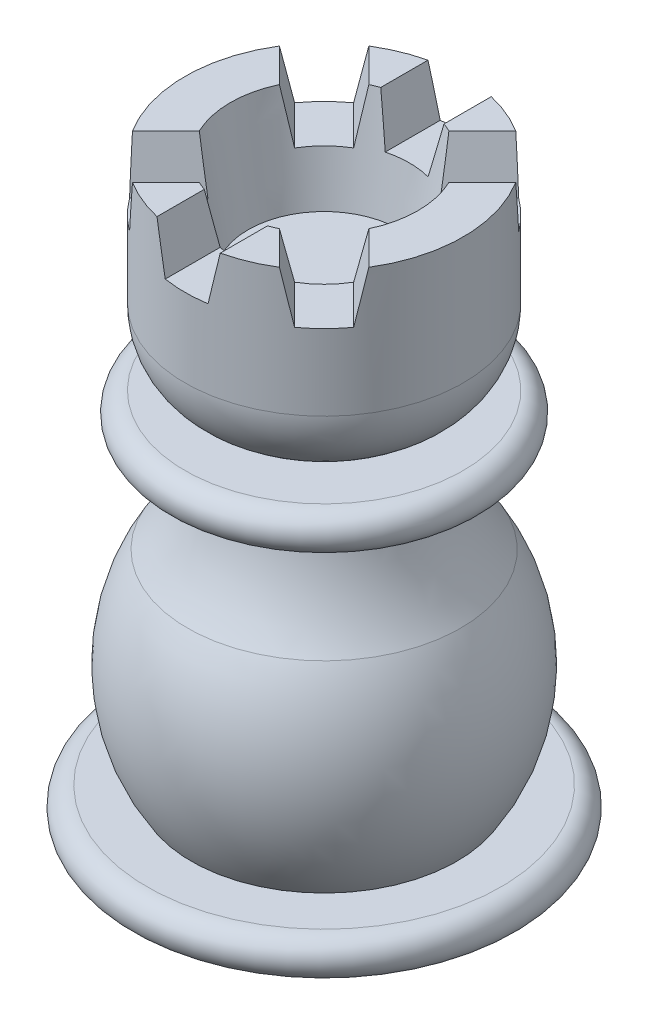
ISO-10303-21;
HEADER;
FILE_DESCRIPTION(('STEP AP214'),'2;1');
FILE_NAME('part.step','',(''),(''),'','','');
FILE_SCHEMA(('AUTOMOTIVE_DESIGN { 1 0 10303 214 1 1 1 1 }'));
ENDSEC;
DATA;
#1=APPLICATION_CONTEXT('core data for automotive mechanical design processes');
#2=APPLICATION_PROTOCOL_DEFINITION('international standard','automotive_design',2000,#1);
#3=PRODUCT_CONTEXT('',#1,'mechanical');
#4=PRODUCT('Part','Part','',(#3));
#5=PRODUCT_RELATED_PRODUCT_CATEGORY('part','',(#4));
#6=PRODUCT_DEFINITION_FORMATION('','',#4);
#7=PRODUCT_DEFINITION_CONTEXT('part definition',#1,'design');
#8=PRODUCT_DEFINITION('design','',#6,#7);
#9=PRODUCT_DEFINITION_SHAPE('','',#8);
#10=(LENGTH_UNIT() NAMED_UNIT(*) SI_UNIT(.MILLI.,.METRE.));
#11=(NAMED_UNIT(*) PLANE_ANGLE_UNIT() SI_UNIT($,.RADIAN.));
#12=(NAMED_UNIT(*) SI_UNIT($,.STERADIAN.) SOLID_ANGLE_UNIT());
#13=UNCERTAINTY_MEASURE_WITH_UNIT(LENGTH_MEASURE(1.E-05),#10,'distance_accuracy_value','');
#14=(GEOMETRIC_REPRESENTATION_CONTEXT(3) GLOBAL_UNCERTAINTY_ASSIGNED_CONTEXT((#13)) GLOBAL_UNIT_ASSIGNED_CONTEXT((#10,
#11,#12)) REPRESENTATION_CONTEXT('',''));
#15=CARTESIAN_POINT('',(0.,0.,0.));
#16=DIRECTION('',(0.,0.,1.));
#17=DIRECTION('',(1.,0.,0.));
#18=AXIS2_PLACEMENT_3D('',#15,#16,#17);
#19=CARTESIAN_POINT('',(0.,46.,0.));
#20=DIRECTION('',(0.,1.,0.));
#21=DIRECTION('',(0.,0.,1.));
#22=AXIS2_PLACEMENT_3D('',#19,#20,#21);
#23=PLANE('',#22);
#24=DIRECTION('',(0.707106781186549,0.,-0.707106781186546));
#25=VECTOR('',#24,1.);
#26=CARTESIAN_POINT('',(-22.9809703885628,46.,26.5165042944955));
#27=LINE('',#26,#25);
#28=CARTESIAN_POINT('',(6.7006782238115,46.,-3.16514431787874));
#29=VERTEX_POINT('',#28);
#30=CARTESIAN_POINT('',(9.34239565673794,46.,-5.80686175080517));
#31=VERTEX_POINT('',#30);
#32=EDGE_CURVE('E359',#29,#31,#27,.T.);
#33=ORIENTED_EDGE('',*,*,#32,.F.);
#34=CARTESIAN_POINT('',(0.,46.,0.));
#35=DIRECTION('',(0.,-1.,0.));
#36=DIRECTION('',(0.,0.,-1.));
#37=AXIS2_PLACEMENT_3D('',#34,#35,#36);
#38=CIRCLE('',#37,7.41061584566773);
#39=CARTESIAN_POINT('',(6.7006782238115,46.,3.16514431787874));
#40=VERTEX_POINT('',#39);
#41=EDGE_CURVE('E290',#29,#40,#38,.T.);
#42=ORIENTED_EDGE('',*,*,#41,.T.);
#43=DIRECTION('',(0.707106781186549,0.,0.707106781186546));
#44=VECTOR('',#43,1.);
#45=CARTESIAN_POINT('',(-22.9809703885629,46.,-26.5165042944955));
#46=LINE('',#45,#44);
#47=CARTESIAN_POINT('',(9.34239565673794,46.,5.80686175080517));
#48=VERTEX_POINT('',#47);
#49=EDGE_CURVE('E228',#40,#48,#46,.T.);
#50=ORIENTED_EDGE('',*,*,#49,.T.);
#51=CARTESIAN_POINT('',(0.,46.,0.));
#52=DIRECTION('',(0.,-1.,0.));
#53=DIRECTION('',(0.,0.,-1.));
#54=AXIS2_PLACEMENT_3D('',#51,#52,#53);
#55=CIRCLE('',#54,11.);
#56=EDGE_CURVE('E322',#31,#48,#55,.T.);
#57=ORIENTED_EDGE('',*,*,#56,.F.);
#58=EDGE_LOOP('',(#33,#42,#50,#57));
#59=FACE_BOUND('',#58,.T.);
#60=ADVANCED_FACE('F41',(#59),#23,.T.);
#61=CARTESIAN_POINT('',(-5.8068617508052,46.,9.34239565673792));
#62=VERTEX_POINT('',#61);
#63=CARTESIAN_POINT('',(-3.16514431787876,46.,6.70067822381149));
#64=VERTEX_POINT('',#63);
#65=EDGE_CURVE('E365',#62,#64,#27,.T.);
#66=ORIENTED_EDGE('',*,*,#65,.F.);
#67=CARTESIAN_POINT('',(-2.5,46.,10.7121426428143));
#68=VERTEX_POINT('',#67);
#69=EDGE_CURVE('E324',#68,#62,#55,.T.);
#70=ORIENTED_EDGE('',*,*,#69,.F.);
#71=DIRECTION('',(0.,0.,1.));
#72=VECTOR('',#71,1.);
#73=CARTESIAN_POINT('',(-2.5,46.,-35.));
#74=LINE('',#73,#72);
#75=CARTESIAN_POINT('',(-2.5,46.,6.97619002121227));
#76=VERTEX_POINT('',#75);
#77=EDGE_CURVE('E253',#76,#68,#74,.T.);
#78=ORIENTED_EDGE('',*,*,#77,.F.);
#79=EDGE_CURVE('E288',#76,#64,#38,.T.);
#80=ORIENTED_EDGE('',*,*,#79,.T.);
#81=EDGE_LOOP('',(#66,#70,#78,#80));
#82=FACE_BOUND('',#81,.T.);
#83=ADVANCED_FACE('F385',(#82),#23,.T.);
#84=CARTESIAN_POINT('',(-5.80686175080522,46.,-9.34239565673791));
#85=VERTEX_POINT('',#84);
#86=CARTESIAN_POINT('',(-3.16514431787878,46.,-6.70067822381148));
#87=VERTEX_POINT('',#86);
#88=EDGE_CURVE('E229',#85,#87,#46,.T.);
#89=ORIENTED_EDGE('',*,*,#88,.T.);
#90=CARTESIAN_POINT('',(-2.5,46.,-6.97619002121227));
#91=VERTEX_POINT('',#90);
#92=EDGE_CURVE('E285',#87,#91,#38,.T.);
#93=ORIENTED_EDGE('',*,*,#92,.T.);
#94=CARTESIAN_POINT('',(-2.5,46.,-10.7121426428143));
#95=VERTEX_POINT('',#94);
#96=EDGE_CURVE('E260',#95,#91,#74,.T.);
#97=ORIENTED_EDGE('',*,*,#96,.F.);
#98=EDGE_CURVE('E317',#85,#95,#55,.T.);
#99=ORIENTED_EDGE('',*,*,#98,.F.);
#100=EDGE_LOOP('',(#89,#93,#97,#99));
#101=FACE_BOUND('',#100,.T.);
#102=ADVANCED_FACE('F406',(#101),#23,.T.);
#103=DIRECTION('',(0.707106781186549,0.,-0.707106781186546));
#104=VECTOR('',#103,1.);
#105=CARTESIAN_POINT('',(-26.5165042944956,46.,22.9809703885628));
#106=LINE('',#105,#104);
#107=CARTESIAN_POINT('',(3.16514431787877,46.,-6.70067822381149));
#108=VERTEX_POINT('',#107);
#109=CARTESIAN_POINT('',(5.80686175080521,46.,-9.34239565673792));
#110=VERTEX_POINT('',#109);
#111=EDGE_CURVE('E63',#108,#110,#106,.T.);
#112=ORIENTED_EDGE('',*,*,#111,.T.);
#113=CARTESIAN_POINT('',(2.5,46.,-10.7121426428143));
#114=VERTEX_POINT('',#113);
#115=EDGE_CURVE('E320',#114,#110,#55,.T.);
#116=ORIENTED_EDGE('',*,*,#115,.F.);
#117=DIRECTION('',(0.,0.,1.));
#118=VECTOR('',#117,1.);
#119=CARTESIAN_POINT('',(2.5,46.,-35.));
#120=LINE('',#119,#118);
#121=CARTESIAN_POINT('',(2.5,46.,-6.9761900212123));
#122=VERTEX_POINT('',#121);
#123=EDGE_CURVE('E259',#114,#122,#120,.T.);
#124=ORIENTED_EDGE('',*,*,#123,.T.);
#125=EDGE_CURVE('E281',#122,#108,#38,.T.);
#126=ORIENTED_EDGE('',*,*,#125,.T.);
#127=EDGE_LOOP('',(#112,#116,#124,#126));
#128=FACE_BOUND('',#127,.T.);
#129=ADVANCED_FACE('F430',(#128),#23,.T.);
#130=CARTESIAN_POINT('',(-9.34239565673793,46.,5.80686175080517));
#131=VERTEX_POINT('',#130);
#132=CARTESIAN_POINT('',(-6.70067822381149,46.,3.16514431787875));
#133=VERTEX_POINT('',#132);
#134=EDGE_CURVE('E203',#131,#133,#106,.T.);
#135=ORIENTED_EDGE('',*,*,#134,.T.);
#136=CARTESIAN_POINT('',(-6.7006782238115,46.,-3.16514431787873));
#137=VERTEX_POINT('',#136);
#138=EDGE_CURVE('E287',#133,#137,#38,.T.);
#139=ORIENTED_EDGE('',*,*,#138,.T.);
#140=DIRECTION('',(0.707106781186549,0.,0.707106781186546));
#141=VECTOR('',#140,1.);
#142=CARTESIAN_POINT('',(-26.5165042944956,46.,-22.9809703885627));
#143=LINE('',#142,#141);
#144=CARTESIAN_POINT('',(-9.34239565673795,46.,-5.80686175080516));
#145=VERTEX_POINT('',#144);
#146=EDGE_CURVE('E243',#145,#137,#143,.T.);
#147=ORIENTED_EDGE('',*,*,#146,.F.);
#148=EDGE_CURVE('E325',#131,#145,#55,.T.);
#149=ORIENTED_EDGE('',*,*,#148,.F.);
#150=EDGE_LOOP('',(#135,#139,#147,#149));
#151=FACE_BOUND('',#150,.T.);
#152=ADVANCED_FACE('F357',(#151),#23,.T.);
#153=CARTESIAN_POINT('',(3.16514431787876,46.,6.70067822381149));
#154=VERTEX_POINT('',#153);
#155=CARTESIAN_POINT('',(5.80686175080521,46.,9.34239565673792));
#156=VERTEX_POINT('',#155);
#157=EDGE_CURVE('E242',#154,#156,#143,.T.);
#158=ORIENTED_EDGE('',*,*,#157,.F.);
#159=CARTESIAN_POINT('',(2.5,46.,6.97619002121231));
#160=VERTEX_POINT('',#159);
#161=EDGE_CURVE('E401',#154,#160,#38,.T.);
#162=ORIENTED_EDGE('',*,*,#161,.T.);
#163=CARTESIAN_POINT('',(2.5,46.,10.7121426428143));
#164=VERTEX_POINT('',#163);
#165=EDGE_CURVE('E256',#160,#164,#120,.T.);
#166=ORIENTED_EDGE('',*,*,#165,.T.);
#167=EDGE_CURVE('E389',#156,#164,#55,.T.);
#168=ORIENTED_EDGE('',*,*,#167,.F.);
#169=EDGE_LOOP('',(#158,#162,#166,#168));
#170=FACE_BOUND('',#169,.T.);
#171=ADVANCED_FACE('F43',(#170),#23,.T.);
#172=CARTESIAN_POINT('',(0.,0.,0.));
#173=DIRECTION('',(0.,-1.,0.));
#174=DIRECTION('',(0.,0.,-1.));
#175=AXIS2_PLACEMENT_3D('',#172,#173,#174);
#176=CYLINDRICAL_SURFACE('',#175,11.);
#177=CARTESIAN_POINT('',(0.,34.2384247263038,0.));
#178=DIRECTION('',(0.691654801480225,-0.207911690817758,0.691654801480227));
#179=DIRECTION('',(-0.147015766465197,-0.978147600733806,-0.147015766465198));
#180=AXIS2_PLACEMENT_3D('',#177,#178,#179);
#181=ELLIPSE('',#180,52.9070777921858,11.);
#182=CARTESIAN_POINT('',(8.85676277814829,42.,-6.52363036135607));
#183=VERTEX_POINT('',#182);
#184=EDGE_CURVE('E234',#31,#183,#181,.F.);
#185=ORIENTED_EDGE('',*,*,#184,.F.);
#186=ORIENTED_EDGE('',*,*,#56,.T.);
#187=CARTESIAN_POINT('',(0.,34.2384247263036,0.));
#188=DIRECTION('',(0.691654801480224,-0.207911690817755,-0.691654801480228));
#189=DIRECTION('',(-0.147015766465195,-0.978147600733806,0.147015766465196));
#190=AXIS2_PLACEMENT_3D('',#187,#188,#189);
#191=ELLIPSE('',#190,52.9070777921864,11.);
#192=CARTESIAN_POINT('',(8.85676277814831,42.,6.52363036135607));
#193=VERTEX_POINT('',#192);
#194=EDGE_CURVE('E251',#193,#48,#191,.F.);
#195=ORIENTED_EDGE('',*,*,#194,.F.);
#196=CARTESIAN_POINT('',(0.,42.,0.));
#197=DIRECTION('',(0.,-1.,0.));
#198=DIRECTION('',(0.,0.,-1.));
#199=AXIS2_PLACEMENT_3D('',#196,#197,#198);
#200=CIRCLE('',#199,11.);
#201=CARTESIAN_POINT('',(6.52363036135612,42.,8.85676277814828));
#202=VERTEX_POINT('',#201);
#203=EDGE_CURVE('E248',#202,#193,#200,.F.);
#204=ORIENTED_EDGE('',*,*,#203,.F.);
#205=CARTESIAN_POINT('',(0.,34.2384247263037,0.));
#206=DIRECTION('',(-0.691654801480224,-0.207911690817758,0.691654801480228));
#207=DIRECTION('',(0.147015766465197,-0.978147600733806,-0.147015766465198));
#208=AXIS2_PLACEMENT_3D('',#205,#206,#207);
#209=ELLIPSE('',#208,52.9070777921858,11.);
#210=EDGE_CURVE('E246',#156,#202,#209,.F.);
#211=ORIENTED_EDGE('',*,*,#210,.F.);
#212=ORIENTED_EDGE('',*,*,#167,.T.);
#213=CARTESIAN_POINT('',(0.,34.2384247263039,0.));
#214=DIRECTION('',(0.978147600733806,-0.20791169081776,0.));
#215=DIRECTION('',(-0.20791169081776,-0.978147600733806,0.));
#216=AXIS2_PLACEMENT_3D('',#213,#214,#215);
#217=ELLIPSE('',#216,52.9070777921853,11.);
#218=CARTESIAN_POINT('',(1.6931281516791,42.203966407899,10.8689151741097));
#219=VERTEX_POINT('',#218);
#220=EDGE_CURVE('E273',#219,#164,#217,.F.);
#221=ORIENTED_EDGE('',*,*,#220,.F.);
#222=CARTESIAN_POINT('',(0.,42.203966407899,0.));
#223=DIRECTION('',(0.,-1.,0.));
#224=DIRECTION('',(1.,0.,0.));
#225=AXIS2_PLACEMENT_3D('',#222,#223,#224);
#226=CIRCLE('',#225,11.);
#227=CARTESIAN_POINT('',(-1.69312815167913,42.203966407899,10.8689151741097));
#228=VERTEX_POINT('',#227);
#229=EDGE_CURVE('E269',#228,#219,#226,.F.);
#230=ORIENTED_EDGE('',*,*,#229,.F.);
#231=CARTESIAN_POINT('',(0.,34.2384247263035,0.));
#232=DIRECTION('',(-0.978147600733807,-0.207911690817753,0.));
#233=DIRECTION('',(0.207911690817753,-0.978147600733807,0.));
#234=AXIS2_PLACEMENT_3D('',#231,#232,#233);
#235=ELLIPSE('',#234,52.9070777921871,11.);
#236=EDGE_CURVE('E277',#68,#228,#235,.F.);
#237=ORIENTED_EDGE('',*,*,#236,.F.);
#238=ORIENTED_EDGE('',*,*,#69,.T.);
#239=CARTESIAN_POINT('',(-6.52363036135611,42.,8.85676277814828));
#240=VERTEX_POINT('',#239);
#241=EDGE_CURVE('E224',#240,#62,#181,.F.);
#242=ORIENTED_EDGE('',*,*,#241,.F.);
#243=CARTESIAN_POINT('',(0.,42.,0.));
#244=DIRECTION('',(0.,-1.,0.));
#245=DIRECTION('',(0.,0.,-1.));
#246=AXIS2_PLACEMENT_3D('',#243,#244,#245);
#247=CIRCLE('',#246,11.);
#248=CARTESIAN_POINT('',(-8.8567627781483,42.,6.52363036135607));
#249=VERTEX_POINT('',#248);
#250=EDGE_CURVE('E211',#249,#240,#247,.F.);
#251=ORIENTED_EDGE('',*,*,#250,.F.);
#252=CARTESIAN_POINT('',(0.,34.2384247263036,0.));
#253=DIRECTION('',(-0.691654801480225,-0.207911690817755,-0.691654801480227));
#254=DIRECTION('',(0.147015766465195,-0.978147600733807,0.147015766465196));
#255=AXIS2_PLACEMENT_3D('',#252,#253,#254);
#256=ELLIPSE('',#255,52.9070777921865,11.);
#257=EDGE_CURVE('E201',#131,#249,#256,.F.);
#258=ORIENTED_EDGE('',*,*,#257,.F.);
#259=ORIENTED_EDGE('',*,*,#148,.T.);
#260=CARTESIAN_POINT('',(-8.8567627781483,42.,-6.52363036135606));
#261=VERTEX_POINT('',#260);
#262=EDGE_CURVE('E247',#261,#145,#209,.F.);
#263=ORIENTED_EDGE('',*,*,#262,.F.);
#264=CARTESIAN_POINT('',(-6.52363036135611,42.,-8.85676277814827));
#265=VERTEX_POINT('',#264);
#266=EDGE_CURVE('E252',#265,#261,#200,.F.);
#267=ORIENTED_EDGE('',*,*,#266,.F.);
#268=EDGE_CURVE('E255',#85,#265,#191,.F.);
#269=ORIENTED_EDGE('',*,*,#268,.F.);
#270=ORIENTED_EDGE('',*,*,#98,.T.);
#271=CARTESIAN_POINT('',(-1.69312815167913,42.203966407899,-10.8689151741097));
#272=VERTEX_POINT('',#271);
#273=EDGE_CURVE('E279',#272,#95,#235,.F.);
#274=ORIENTED_EDGE('',*,*,#273,.F.);
#275=CARTESIAN_POINT('',(1.6931281516791,42.203966407899,-10.8689151741097));
#276=VERTEX_POINT('',#275);
#277=EDGE_CURVE('E275',#276,#272,#226,.F.);
#278=ORIENTED_EDGE('',*,*,#277,.F.);
#279=EDGE_CURVE('E271',#114,#276,#217,.F.);
#280=ORIENTED_EDGE('',*,*,#279,.F.);
#281=ORIENTED_EDGE('',*,*,#115,.T.);
#282=CARTESIAN_POINT('',(6.5236303613561,42.,-8.85676277814828));
#283=VERTEX_POINT('',#282);
#284=EDGE_CURVE('E206',#283,#110,#256,.F.);
#285=ORIENTED_EDGE('',*,*,#284,.F.);
#286=EDGE_CURVE('E227',#183,#283,#247,.F.);
#287=ORIENTED_EDGE('',*,*,#286,.F.);
#288=EDGE_LOOP('',(#185,#186,#195,#204,#211,#212,#221,#230,#237,#238,#242,#251,#258,#259,#263,
#267,#269,#270,#274,#278,#280,#281,#285,#287));
#289=FACE_BOUND('',#288,.T.);
#290=CARTESIAN_POINT('',(0.,36.,0.));
#291=DIRECTION('',(0.,-1.,0.));
#292=DIRECTION('',(0.,0.,-1.));
#293=AXIS2_PLACEMENT_3D('',#290,#291,#292);
#294=CIRCLE('',#293,11.);
#295=CARTESIAN_POINT('',(0.,36.,-11.));
#296=VERTEX_POINT('',#295);
#297=EDGE_CURVE('E312',#296,#296,#294,.T.);
#298=ORIENTED_EDGE('',*,*,#297,.F.);
#299=EDGE_LOOP('',(#298));
#300=FACE_BOUND('',#299,.T.);
#301=ADVANCED_FACE('F225',(#289,#300),#176,.T.);
#302=CARTESIAN_POINT('',(0.,36.,0.));
#303=DIRECTION('',(0.,-1.,0.));
#304=DIRECTION('',(0.,0.,-1.));
#305=AXIS2_PLACEMENT_3D('',#302,#303,#304);
#306=DEGENERATE_TOROIDAL_SURFACE('',#305,5.,6.,.T.);
#307=ORIENTED_EDGE('',*,*,#297,.T.);
#308=EDGE_LOOP('',(#307));
#309=FACE_BOUND('',#308,.T.);
#310=CARTESIAN_POINT('',(0.,30.,0.));
#311=DIRECTION('',(0.,-1.,0.));
#312=DIRECTION('',(0.,0.,-1.));
#313=AXIS2_PLACEMENT_3D('',#310,#311,#312);
#314=CIRCLE('',#313,5.);
#315=CARTESIAN_POINT('',(0.,30.,-5.));
#316=VERTEX_POINT('',#315);
#317=EDGE_CURVE('E309',#316,#316,#314,.T.);
#318=ORIENTED_EDGE('',*,*,#317,.F.);
#319=EDGE_LOOP('',(#318));
#320=FACE_BOUND('',#319,.T.);
#321=ADVANCED_FACE('F443',(#309,#320),#306,.T.);
#322=CARTESIAN_POINT('',(0.,30.,0.));
#323=DIRECTION('',(0.,1.,0.));
#324=DIRECTION('',(0.,0.,1.));
#325=AXIS2_PLACEMENT_3D('',#322,#323,#324);
#326=PLANE('',#325);
#327=ORIENTED_EDGE('',*,*,#317,.T.);
#328=EDGE_LOOP('',(#327));
#329=FACE_BOUND('',#328,.T.);
#330=CARTESIAN_POINT('',(0.,30.,0.));
#331=DIRECTION('',(0.,-1.,0.));
#332=DIRECTION('',(0.,0.,-1.));
#333=AXIS2_PLACEMENT_3D('',#330,#331,#332);
#334=CIRCLE('',#333,11.);
#335=CARTESIAN_POINT('',(0.,30.,-11.));
#336=VERTEX_POINT('',#335);
#337=EDGE_CURVE('E310',#336,#336,#334,.T.);
#338=ORIENTED_EDGE('',*,*,#337,.F.);
#339=EDGE_LOOP('',(#338));
#340=FACE_BOUND('',#339,.T.);
#341=ADVANCED_FACE('F715',(#329,#340),#326,.T.);
#342=CARTESIAN_POINT('',(0.,28.5,0.));
#343=DIRECTION('',(0.,-1.,0.));
#344=DIRECTION('',(0.,0.,-1.));
#345=AXIS2_PLACEMENT_3D('',#342,#343,#344);
#346=TOROIDAL_SURFACE('',#345,11.,1.5);
#347=CARTESIAN_POINT('',(0.,27.,0.));
#348=DIRECTION('',(0.,-1.,0.));
#349=DIRECTION('',(0.,0.,-1.));
#350=AXIS2_PLACEMENT_3D('',#347,#348,#349);
#351=CIRCLE('',#350,11.);
#352=CARTESIAN_POINT('',(0.,27.,-11.));
#353=VERTEX_POINT('',#352);
#354=EDGE_CURVE('E302',#353,#353,#351,.T.);
#355=ORIENTED_EDGE('',*,*,#354,.F.);
#356=EDGE_LOOP('',(#355));
#357=FACE_BOUND('',#356,.T.);
#358=ORIENTED_EDGE('',*,*,#337,.T.);
#359=EDGE_LOOP('',(#358));
#360=FACE_BOUND('',#359,.T.);
#361=ADVANCED_FACE('F702',(#357,#360),#346,.T.);
#362=CARTESIAN_POINT('',(0.,27.,0.));
#363=DIRECTION('',(0.,1.,0.));
#364=DIRECTION('',(0.,0.,1.));
#365=AXIS2_PLACEMENT_3D('',#362,#363,#364);
#366=PLANE('',#365);
#367=CARTESIAN_POINT('',(0.,27.,0.));
#368=DIRECTION('',(0.,-1.,0.));
#369=DIRECTION('',(0.,0.,-1.));
#370=AXIS2_PLACEMENT_3D('',#367,#368,#369);
#371=CIRCLE('',#370,8.00000000000001);
#372=CARTESIAN_POINT('',(0.,27.,-8.00000000000001));
#373=VERTEX_POINT('',#372);
#374=EDGE_CURVE('E301',#373,#373,#371,.T.);
#375=ORIENTED_EDGE('',*,*,#374,.F.);
#376=EDGE_LOOP('',(#375));
#377=FACE_BOUND('',#376,.T.);
#378=ORIENTED_EDGE('',*,*,#354,.T.);
#379=EDGE_LOOP('',(#378));
#380=FACE_BOUND('',#379,.T.);
#381=ADVANCED_FACE('F692',(#377,#380),#366,.F.);
#382=CARTESIAN_POINT('',(0.,27.8746859276655,0.));
#383=DIRECTION('',(0.,-1.,0.));
#384=DIRECTION('',(0.,0.,-1.));
#385=AXIS2_PLACEMENT_3D('',#382,#383,#384);
#386=TOROIDAL_SURFACE('',#385,22.9744757680509,15.);
#387=ORIENTED_EDGE('',*,*,#374,.T.);
#388=EDGE_LOOP('',(#387));
#389=FACE_BOUND('',#388,.T.);
#390=CARTESIAN_POINT('',(0.,19.112684674635,0.));
#391=DIRECTION('',(0.,-1.,0.));
#392=DIRECTION('',(0.,0.,-1.));
#393=AXIS2_PLACEMENT_3D('',#390,#391,#392);
#394=CIRCLE('',#393,10.7996109210847);
#395=CARTESIAN_POINT('',(0.,19.112684674635,-10.7996109210847));
#396=VERTEX_POINT('',#395);
#397=EDGE_CURVE('E296',#396,#396,#394,.T.);
#398=ORIENTED_EDGE('',*,*,#397,.F.);
#399=EDGE_LOOP('',(#398));
#400=FACE_BOUND('',#399,.T.);
#401=ADVANCED_FACE('F685',(#389,#400),#386,.F.);
#402=CARTESIAN_POINT('',(0.,11.2915619758885,0.));
#403=DIRECTION('',(0.,-1.,0.));
#404=DIRECTION('',(0.,0.,-1.));
#405=AXIS2_PLACEMENT_3D('',#402,#403,#404);
#406=DEGENERATE_TOROIDAL_SURFACE('',#405,2.,15.,.F.);
#407=CARTESIAN_POINT('',(0.,3.,0.));
#408=DIRECTION('',(0.,-1.,0.));
#409=DIRECTION('',(0.,0.,-1.));
#410=AXIS2_PLACEMENT_3D('',#407,#408,#409);
#411=CIRCLE('',#410,10.5);
#412=CARTESIAN_POINT('',(0.,3.,-10.5));
#413=VERTEX_POINT('',#412);
#414=EDGE_CURVE('E294',#413,#413,#411,.T.);
#415=ORIENTED_EDGE('',*,*,#414,.F.);
#416=EDGE_LOOP('',(#415));
#417=FACE_BOUND('',#416,.T.);
#418=ORIENTED_EDGE('',*,*,#397,.T.);
#419=EDGE_LOOP('',(#418));
#420=FACE_BOUND('',#419,.T.);
#421=ADVANCED_FACE('F674',(#417,#420),#406,.F.);
#422=CARTESIAN_POINT('',(0.,3.,0.));
#423=DIRECTION('',(0.,1.,0.));
#424=DIRECTION('',(0.,0.,1.));
#425=AXIS2_PLACEMENT_3D('',#422,#423,#424);
#426=PLANE('',#425);
#427=ORIENTED_EDGE('',*,*,#414,.T.);
#428=EDGE_LOOP('',(#427));
#429=FACE_BOUND('',#428,.T.);
#430=CARTESIAN_POINT('',(0.,3.,0.));
#431=DIRECTION('',(0.,-1.,0.));
#432=DIRECTION('',(0.,0.,-1.));
#433=AXIS2_PLACEMENT_3D('',#430,#431,#432);
#434=CIRCLE('',#433,14.);
#435=CARTESIAN_POINT('',(0.,3.,-14.));
#436=VERTEX_POINT('',#435);
#437=EDGE_CURVE('E292',#436,#436,#434,.T.);
#438=ORIENTED_EDGE('',*,*,#437,.F.);
#439=EDGE_LOOP('',(#438));
#440=FACE_BOUND('',#439,.T.);
#441=ADVANCED_FACE('F667',(#429,#440),#426,.T.);
#442=CARTESIAN_POINT('',(0.,1.5,0.));
#443=DIRECTION('',(0.,-1.,0.));
#444=DIRECTION('',(0.,0.,-1.));
#445=AXIS2_PLACEMENT_3D('',#442,#443,#444);
#446=TOROIDAL_SURFACE('',#445,14.,1.5);
#447=CARTESIAN_POINT('',(0.,0.,0.));
#448=DIRECTION('',(0.,-1.,0.));
#449=DIRECTION('',(0.,0.,-1.));
#450=AXIS2_PLACEMENT_3D('',#447,#448,#449);
#451=CIRCLE('',#450,14.);
#452=CARTESIAN_POINT('',(0.,0.,-14.));
#453=VERTEX_POINT('',#452);
#454=EDGE_CURVE('E286',#453,#453,#451,.T.);
#455=ORIENTED_EDGE('',*,*,#454,.F.);
#456=EDGE_LOOP('',(#455));
#457=FACE_BOUND('',#456,.T.);
#458=ORIENTED_EDGE('',*,*,#437,.T.);
#459=EDGE_LOOP('',(#458));
#460=FACE_BOUND('',#459,.T.);
#461=ADVANCED_FACE('F656',(#457,#460),#446,.T.);
#462=CARTESIAN_POINT('',(0.,0.,0.));
#463=DIRECTION('',(0.,1.,0.));
#464=DIRECTION('',(0.,0.,1.));
#465=AXIS2_PLACEMENT_3D('',#462,#463,#464);
#466=PLANE('',#465);
#467=ORIENTED_EDGE('',*,*,#454,.T.);
#468=EDGE_LOOP('',(#467));
#469=FACE_BOUND('',#468,.T.);
#470=ADVANCED_FACE('F649',(#469),#466,.F.);
#471=CARTESIAN_POINT('',(0.,38.,0.));
#472=DIRECTION('',(0.,1.,0.));
#473=DIRECTION('',(0.,0.,1.));
#474=AXIS2_PLACEMENT_3D('',#471,#472,#473);
#475=CONICAL_SURFACE('',#474,6.,0.174532925199434);
#476=CARTESIAN_POINT('',(0.,42.,0.));
#477=DIRECTION('',(0.,-1.,0.));
#478=DIRECTION('',(0.,0.,-1.));
#479=AXIS2_PLACEMENT_3D('',#476,#477,#478);
#480=CIRCLE('',#479,6.70530792283387);
#481=CARTESIAN_POINT('',(-5.76218373506623,42.,3.42905131827402));
#482=VERTEX_POINT('',#481);
#483=CARTESIAN_POINT('',(-3.42905131827403,42.,5.76218373506622));
#484=VERTEX_POINT('',#483);
#485=EDGE_CURVE('E49',#482,#484,#480,.F.);
#486=ORIENTED_EDGE('',*,*,#485,.T.);
#487=CARTESIAN_POINT('',(10.0385473686696,101.028410995166,10.0385473686696));
#488=DIRECTION('',(0.691654801480225,-0.207911690817758,0.691654801480227));
#489=DIRECTION('',(0.147015766465197,0.978147600733806,0.147015766465198));
#490=AXIS2_PLACEMENT_3D('',#487,#488,#489);
#491=ELLIPSE('',#490,82.3119149400342,9.55671284905689);
#492=EDGE_CURVE('E11',#484,#64,#491,.F.);
#493=ORIENTED_EDGE('',*,*,#492,.T.);
#494=ORIENTED_EDGE('',*,*,#79,.F.);
#495=CARTESIAN_POINT('',(-14.1966498352994,101.028410995177,0.));
#496=DIRECTION('',(-0.978147600733807,-0.207911690817753,0.));
#497=DIRECTION('',(-0.207911690817753,0.978147600733807,0.));
#498=AXIS2_PLACEMENT_3D('',#495,#496,#497);
#499=ELLIPSE('',#498,82.3119149400463,9.55671284905743);
#500=CARTESIAN_POINT('',(-1.69312815167913,42.203966407899,6.5251877158979));
#501=VERTEX_POINT('',#500);
#502=EDGE_CURVE('E329',#76,#501,#499,.F.);
#503=ORIENTED_EDGE('',*,*,#502,.T.);
#504=CARTESIAN_POINT('',(0.,42.203966407899,0.));
#505=DIRECTION('',(0.,-1.,0.));
#506=DIRECTION('',(1.,0.,0.));
#507=AXIS2_PLACEMENT_3D('',#504,#505,#506);
#508=CIRCLE('',#507,6.74127270370464);
#509=CARTESIAN_POINT('',(1.6931281516791,42.203966407899,6.52518771589792));
#510=VERTEX_POINT('',#509);
#511=EDGE_CURVE('E318',#501,#510,#508,.F.);
#512=ORIENTED_EDGE('',*,*,#511,.T.);
#513=CARTESIAN_POINT('',(14.1966498352967,101.028410995163,0.));
#514=DIRECTION('',(0.978147600733806,-0.20791169081776,0.));
#515=DIRECTION('',(0.20791169081776,0.978147600733805,0.));
#516=AXIS2_PLACEMENT_3D('',#513,#514,#515);
#517=ELLIPSE('',#516,82.3119149400311,9.55671284905677);
#518=EDGE_CURVE('E328',#510,#160,#517,.F.);
#519=ORIENTED_EDGE('',*,*,#518,.T.);
#520=ORIENTED_EDGE('',*,*,#161,.F.);
#521=CARTESIAN_POINT('',(-10.0385473686697,101.028410995167,10.0385473686698));
#522=DIRECTION('',(-0.691654801480224,-0.207911690817758,0.691654801480228));
#523=DIRECTION('',(-0.147015766465197,0.978147600733806,0.147015766465198));
#524=AXIS2_PLACEMENT_3D('',#521,#522,#523);
#525=ELLIPSE('',#524,82.3119149400355,9.55671284905696);
#526=CARTESIAN_POINT('',(3.42905131827407,42.,5.76218373506625));
#527=VERTEX_POINT('',#526);
#528=EDGE_CURVE('E339',#154,#527,#525,.F.);
#529=ORIENTED_EDGE('',*,*,#528,.T.);
#530=CARTESIAN_POINT('',(0.,42.,0.));
#531=DIRECTION('',(0.,-1.,0.));
#532=DIRECTION('',(0.,0.,-1.));
#533=AXIS2_PLACEMENT_3D('',#530,#531,#532);
#534=CIRCLE('',#533,6.70530792283387);
#535=CARTESIAN_POINT('',(5.76218373506623,42.,3.42905131827401));
#536=VERTEX_POINT('',#535);
#537=EDGE_CURVE('E344',#527,#536,#534,.F.);
#538=ORIENTED_EDGE('',*,*,#537,.T.);
#539=CARTESIAN_POINT('',(10.0385473686704,101.028410995173,-10.0385473686705));
#540=DIRECTION('',(0.691654801480224,-0.207911690817755,-0.691654801480228));
#541=DIRECTION('',(0.147015766465195,0.978147600733807,-0.147015766465196));
#542=AXIS2_PLACEMENT_3D('',#539,#540,#541);
#543=ELLIPSE('',#542,82.3119149400413,9.55671284905723);
#544=EDGE_CURVE('E348',#536,#40,#543,.F.);
#545=ORIENTED_EDGE('',*,*,#544,.T.);
#546=ORIENTED_EDGE('',*,*,#41,.F.);
#547=CARTESIAN_POINT('',(5.76218373506623,42.,-3.42905131827402));
#548=VERTEX_POINT('',#547);
#549=EDGE_CURVE('E44',#29,#548,#491,.F.);
#550=ORIENTED_EDGE('',*,*,#549,.T.);
#551=CARTESIAN_POINT('',(3.42905131827404,42.,-5.76218373506623));
#552=VERTEX_POINT('',#551);
#553=EDGE_CURVE('E346',#548,#552,#480,.F.);
#554=ORIENTED_EDGE('',*,*,#553,.T.);
#555=CARTESIAN_POINT('',(-10.0385473686703,101.028410995172,-10.0385473686703));
#556=DIRECTION('',(-0.691654801480225,-0.207911690817755,-0.691654801480227));
#557=DIRECTION('',(-0.147015766465195,0.978147600733807,-0.147015766465196));
#558=AXIS2_PLACEMENT_3D('',#555,#556,#557);
#559=ELLIPSE('',#558,82.3119149400398,9.55671284905713);
#560=EDGE_CURVE('E350',#552,#108,#559,.F.);
#561=ORIENTED_EDGE('',*,*,#560,.T.);
#562=ORIENTED_EDGE('',*,*,#125,.F.);
#563=CARTESIAN_POINT('',(1.6931281516791,42.203966407899,-6.52518771589792));
#564=VERTEX_POINT('',#563);
#565=EDGE_CURVE('E331',#122,#564,#517,.F.);
#566=ORIENTED_EDGE('',*,*,#565,.T.);
#567=CARTESIAN_POINT('',(-1.69312815167913,42.203966407899,-6.5251877158979));
#568=VERTEX_POINT('',#567);
#569=EDGE_CURVE('E330',#564,#568,#508,.F.);
#570=ORIENTED_EDGE('',*,*,#569,.T.);
#571=EDGE_CURVE('E333',#568,#91,#499,.F.);
#572=ORIENTED_EDGE('',*,*,#571,.T.);
#573=ORIENTED_EDGE('',*,*,#92,.F.);
#574=CARTESIAN_POINT('',(-3.42905131827405,42.,-5.76218373506622));
#575=VERTEX_POINT('',#574);
#576=EDGE_CURVE('E345',#87,#575,#543,.F.);
#577=ORIENTED_EDGE('',*,*,#576,.T.);
#578=CARTESIAN_POINT('',(-5.76218373506626,42.,-3.42905131827403));
#579=VERTEX_POINT('',#578);
#580=EDGE_CURVE('E336',#575,#579,#534,.F.);
#581=ORIENTED_EDGE('',*,*,#580,.T.);
#582=EDGE_CURVE('E334',#579,#137,#525,.F.);
#583=ORIENTED_EDGE('',*,*,#582,.T.);
#584=ORIENTED_EDGE('',*,*,#138,.F.);
#585=EDGE_CURVE('E347',#133,#482,#559,.F.);
#586=ORIENTED_EDGE('',*,*,#585,.T.);
#587=EDGE_LOOP('',(#486,#493,#494,#503,#512,#519,#520,#529,#538,#545,#546,#550,#554,#561,#562,
#566,#570,#572,#573,#577,#581,#583,#584,#586));
#588=FACE_BOUND('',#587,.T.);
#589=CARTESIAN_POINT('',(0.,38.,0.));
#590=DIRECTION('',(0.,-1.,0.));
#591=DIRECTION('',(0.,0.,-1.));
#592=AXIS2_PLACEMENT_3D('',#589,#590,#591);
#593=CIRCLE('',#592,6.);
#594=CARTESIAN_POINT('',(0.,38.,-6.));
#595=VERTEX_POINT('',#594);
#596=EDGE_CURVE('E276',#595,#595,#593,.T.);
#597=ORIENTED_EDGE('',*,*,#596,.T.);
#598=EDGE_LOOP('',(#597));
#599=FACE_BOUND('',#598,.T.);
#600=ADVANCED_FACE('F353',(#588,#599),#475,.F.);
#601=CARTESIAN_POINT('',(0.,38.,0.));
#602=DIRECTION('',(0.,-1.,0.));
#603=DIRECTION('',(0.,0.,-1.));
#604=AXIS2_PLACEMENT_3D('',#601,#602,#603);
#605=PLANE('',#604);
#606=ORIENTED_EDGE('',*,*,#596,.F.);
#607=EDGE_LOOP('',(#606));
#608=FACE_BOUND('',#607,.T.);
#609=ADVANCED_FACE('F498',(#608),#605,.F.);
#610=CARTESIAN_POINT('',(1.6931281516791,42.203966407899,-35.));
#611=DIRECTION('',(0.,-1.,0.));
#612=DIRECTION('',(1.,0.,0.));
#613=AXIS2_PLACEMENT_3D('',#610,#611,#612);
#614=PLANE('',#613);
#615=ORIENTED_EDGE('',*,*,#229,.T.);
#616=DIRECTION('',(0.,0.,1.));
#617=VECTOR('',#616,1.);
#618=CARTESIAN_POINT('',(1.6931281516791,42.203966407899,-35.));
#619=LINE('',#618,#617);
#620=EDGE_CURVE('E261',#510,#219,#619,.T.);
#621=ORIENTED_EDGE('',*,*,#620,.F.);
#622=ORIENTED_EDGE('',*,*,#511,.F.);
#623=DIRECTION('',(0.,0.,1.));
#624=VECTOR('',#623,1.);
#625=CARTESIAN_POINT('',(-1.69312815167913,42.203966407899,-35.));
#626=LINE('',#625,#624);
#627=EDGE_CURVE('E270',#501,#228,#626,.T.);
#628=ORIENTED_EDGE('',*,*,#627,.T.);
#629=EDGE_LOOP('',(#615,#621,#622,#628));
#630=FACE_BOUND('',#629,.T.);
#631=ADVANCED_FACE('F493',(#630),#614,.F.);
#632=CARTESIAN_POINT('',(2.5,46.,-35.));
#633=DIRECTION('',(0.978147600733806,-0.20791169081776,0.));
#634=DIRECTION('',(0.20791169081776,0.978147600733806,0.));
#635=AXIS2_PLACEMENT_3D('',#632,#633,#634);
#636=PLANE('',#635);
#637=ORIENTED_EDGE('',*,*,#220,.T.);
#638=ORIENTED_EDGE('',*,*,#165,.F.);
#639=ORIENTED_EDGE('',*,*,#518,.F.);
#640=ORIENTED_EDGE('',*,*,#620,.T.);
#641=EDGE_LOOP('',(#637,#638,#639,#640));
#642=FACE_BOUND('',#641,.T.);
#643=ADVANCED_FACE('F458',(#642),#636,.F.);
#644=CARTESIAN_POINT('',(-1.69312815167913,42.203966407899,-35.));
#645=DIRECTION('',(-0.978147600733807,-0.207911690817753,0.));
#646=DIRECTION('',(0.207911690817753,-0.978147600733807,0.));
#647=AXIS2_PLACEMENT_3D('',#644,#645,#646);
#648=PLANE('',#647);
#649=ORIENTED_EDGE('',*,*,#236,.T.);
#650=ORIENTED_EDGE('',*,*,#627,.F.);
#651=ORIENTED_EDGE('',*,*,#502,.F.);
#652=ORIENTED_EDGE('',*,*,#77,.T.);
#653=EDGE_LOOP('',(#649,#650,#651,#652));
#654=FACE_BOUND('',#653,.T.);
#655=ADVANCED_FACE('F502',(#654),#648,.F.);
#656=ORIENTED_EDGE('',*,*,#273,.T.);
#657=ORIENTED_EDGE('',*,*,#96,.T.);
#658=ORIENTED_EDGE('',*,*,#571,.F.);
#659=EDGE_CURVE('E266',#272,#568,#626,.T.);
#660=ORIENTED_EDGE('',*,*,#659,.F.);
#661=EDGE_LOOP('',(#656,#657,#658,#660));
#662=FACE_BOUND('',#661,.T.);
#663=ADVANCED_FACE('F414',(#662),#648,.F.);
#664=ORIENTED_EDGE('',*,*,#279,.T.);
#665=EDGE_CURVE('E265',#276,#564,#619,.T.);
#666=ORIENTED_EDGE('',*,*,#665,.T.);
#667=ORIENTED_EDGE('',*,*,#565,.F.);
#668=ORIENTED_EDGE('',*,*,#123,.F.);
#669=EDGE_LOOP('',(#664,#666,#667,#668));
#670=FACE_BOUND('',#669,.T.);
#671=ADVANCED_FACE('F425',(#670),#636,.F.);
#672=ORIENTED_EDGE('',*,*,#277,.T.);
#673=ORIENTED_EDGE('',*,*,#659,.T.);
#674=ORIENTED_EDGE('',*,*,#569,.F.);
#675=ORIENTED_EDGE('',*,*,#665,.F.);
#676=EDGE_LOOP('',(#672,#673,#674,#675));
#677=FACE_BOUND('',#676,.T.);
#678=ADVANCED_FACE('F477',(#677),#614,.F.);
#679=CARTESIAN_POINT('',(-26.5165042944956,46.,-22.9809703885627));
#680=DIRECTION('',(-0.691654801480224,-0.207911690817758,0.691654801480228));
#681=DIRECTION('',(0.707106781186549,0.,0.707106781186546));
#682=AXIS2_PLACEMENT_3D('',#679,#680,#681);
#683=PLANE('',#682);
#684=ORIENTED_EDGE('',*,*,#262,.T.);
#685=ORIENTED_EDGE('',*,*,#146,.T.);
#686=ORIENTED_EDGE('',*,*,#582,.F.);
#687=DIRECTION('',(0.707106781186549,0.,0.707106781186546));
#688=VECTOR('',#687,1.);
#689=CARTESIAN_POINT('',(-25.9153035499253,42.,-23.582171133133));
#690=LINE('',#689,#688);
#691=EDGE_CURVE('E237',#261,#579,#690,.T.);
#692=ORIENTED_EDGE('',*,*,#691,.F.);
#693=EDGE_LOOP('',(#684,#685,#686,#692));
#694=FACE_BOUND('',#693,.T.);
#695=ADVANCED_FACE('F469',(#694),#683,.F.);
#696=CARTESIAN_POINT('',(-25.9153035499253,42.,-23.582171133133));
#697=DIRECTION('',(0.,-1.,0.));
#698=DIRECTION('',(0.,0.,-1.));
#699=AXIS2_PLACEMENT_3D('',#696,#697,#698);
#700=PLANE('',#699);
#701=ORIENTED_EDGE('',*,*,#266,.T.);
#702=ORIENTED_EDGE('',*,*,#691,.T.);
#703=ORIENTED_EDGE('',*,*,#580,.F.);
#704=DIRECTION('',(0.707106781186549,0.,0.707106781186546));
#705=VECTOR('',#704,1.);
#706=CARTESIAN_POINT('',(-23.5821711331331,42.,-25.9153035499252));
#707=LINE('',#706,#705);
#708=EDGE_CURVE('E238',#265,#575,#707,.T.);
#709=ORIENTED_EDGE('',*,*,#708,.F.);
#710=EDGE_LOOP('',(#701,#702,#703,#709));
#711=FACE_BOUND('',#710,.T.);
#712=ADVANCED_FACE('F463',(#711),#700,.F.);
#713=CARTESIAN_POINT('',(-23.5821711331331,42.,-25.9153035499252));
#714=DIRECTION('',(0.691654801480224,-0.207911690817755,-0.691654801480228));
#715=DIRECTION('',(-0.707106781186549,0.,-0.707106781186546));
#716=AXIS2_PLACEMENT_3D('',#713,#714,#715);
#717=PLANE('',#716);
#718=ORIENTED_EDGE('',*,*,#268,.T.);
#719=ORIENTED_EDGE('',*,*,#708,.T.);
#720=ORIENTED_EDGE('',*,*,#576,.F.);
#721=ORIENTED_EDGE('',*,*,#88,.F.);
#722=EDGE_LOOP('',(#718,#719,#720,#721));
#723=FACE_BOUND('',#722,.T.);
#724=ADVANCED_FACE('F468',(#723),#717,.F.);
#725=ORIENTED_EDGE('',*,*,#194,.T.);
#726=ORIENTED_EDGE('',*,*,#49,.F.);
#727=ORIENTED_EDGE('',*,*,#544,.F.);
#728=EDGE_CURVE('E232',#536,#193,#707,.T.);
#729=ORIENTED_EDGE('',*,*,#728,.T.);
#730=EDGE_LOOP('',(#725,#726,#727,#729));
#731=FACE_BOUND('',#730,.T.);
#732=ADVANCED_FACE('F398',(#731),#717,.F.);
#733=ORIENTED_EDGE('',*,*,#203,.T.);
#734=ORIENTED_EDGE('',*,*,#728,.F.);
#735=ORIENTED_EDGE('',*,*,#537,.F.);
#736=EDGE_CURVE('E239',#527,#202,#690,.T.);
#737=ORIENTED_EDGE('',*,*,#736,.T.);
#738=EDGE_LOOP('',(#733,#734,#735,#737));
#739=FACE_BOUND('',#738,.T.);
#740=ADVANCED_FACE('F461',(#739),#700,.F.);
#741=ORIENTED_EDGE('',*,*,#210,.T.);
#742=ORIENTED_EDGE('',*,*,#736,.F.);
#743=ORIENTED_EDGE('',*,*,#528,.F.);
#744=ORIENTED_EDGE('',*,*,#157,.T.);
#745=EDGE_LOOP('',(#741,#742,#743,#744));
#746=FACE_BOUND('',#745,.T.);
#747=ADVANCED_FACE('F456',(#746),#683,.F.);
#748=CARTESIAN_POINT('',(-25.9153035499253,42.,23.582171133133));
#749=DIRECTION('',(-0.691654801480225,-0.207911690817755,-0.691654801480227));
#750=DIRECTION('',(-0.707106781186549,0.,0.707106781186546));
#751=AXIS2_PLACEMENT_3D('',#748,#749,#750);
#752=PLANE('',#751);
#753=ORIENTED_EDGE('',*,*,#284,.T.);
#754=ORIENTED_EDGE('',*,*,#111,.F.);
#755=ORIENTED_EDGE('',*,*,#560,.F.);
#756=DIRECTION('',(0.707106781186549,0.,-0.707106781186546));
#757=VECTOR('',#756,1.);
#758=CARTESIAN_POINT('',(-25.9153035499253,42.,23.582171133133));
#759=LINE('',#758,#757);
#760=EDGE_CURVE('E216',#552,#283,#759,.T.);
#761=ORIENTED_EDGE('',*,*,#760,.T.);
#762=EDGE_LOOP('',(#753,#754,#755,#761));
#763=FACE_BOUND('',#762,.T.);
#764=ADVANCED_FACE('F368',(#763),#752,.F.);
#765=CARTESIAN_POINT('',(-22.9809703885628,46.,26.5165042944955));
#766=DIRECTION('',(0.691654801480225,-0.207911690817758,0.691654801480227));
#767=DIRECTION('',(0.707106781186549,0.,-0.707106781186547));
#768=AXIS2_PLACEMENT_3D('',#765,#766,#767);
#769=PLANE('',#768);
#770=ORIENTED_EDGE('',*,*,#184,.T.);
#771=DIRECTION('',(0.707106781186549,0.,-0.707106781186546));
#772=VECTOR('',#771,1.);
#773=CARTESIAN_POINT('',(-23.5821711331331,42.,25.9153035499252));
#774=LINE('',#773,#772);
#775=EDGE_CURVE('E383',#548,#183,#774,.T.);
#776=ORIENTED_EDGE('',*,*,#775,.F.);
#777=ORIENTED_EDGE('',*,*,#549,.F.);
#778=ORIENTED_EDGE('',*,*,#32,.T.);
#779=EDGE_LOOP('',(#770,#776,#777,#778));
#780=FACE_BOUND('',#779,.T.);
#781=ADVANCED_FACE('F509',(#780),#769,.F.);
#782=CARTESIAN_POINT('',(-23.5821711331331,42.,25.9153035499252));
#783=DIRECTION('',(0.,-1.,0.));
#784=DIRECTION('',(0.,0.,-1.));
#785=AXIS2_PLACEMENT_3D('',#782,#783,#784);
#786=PLANE('',#785);
#787=ORIENTED_EDGE('',*,*,#286,.T.);
#788=ORIENTED_EDGE('',*,*,#760,.F.);
#789=ORIENTED_EDGE('',*,*,#553,.F.);
#790=ORIENTED_EDGE('',*,*,#775,.T.);
#791=EDGE_LOOP('',(#787,#788,#789,#790));
#792=FACE_BOUND('',#791,.T.);
#793=ADVANCED_FACE('F508',(#792),#786,.F.);
#794=ORIENTED_EDGE('',*,*,#250,.T.);
#795=EDGE_CURVE('E209',#240,#484,#774,.T.);
#796=ORIENTED_EDGE('',*,*,#795,.T.);
#797=ORIENTED_EDGE('',*,*,#485,.F.);
#798=EDGE_CURVE('E60',#249,#482,#759,.T.);
#799=ORIENTED_EDGE('',*,*,#798,.F.);
#800=EDGE_LOOP('',(#794,#796,#797,#799));
#801=FACE_BOUND('',#800,.T.);
#802=ADVANCED_FACE('F215',(#801),#786,.F.);
#803=ORIENTED_EDGE('',*,*,#241,.T.);
#804=ORIENTED_EDGE('',*,*,#65,.T.);
#805=ORIENTED_EDGE('',*,*,#492,.F.);
#806=ORIENTED_EDGE('',*,*,#795,.F.);
#807=EDGE_LOOP('',(#803,#804,#805,#806));
#808=FACE_BOUND('',#807,.T.);
#809=ADVANCED_FACE('F377',(#808),#769,.F.);
#810=ORIENTED_EDGE('',*,*,#257,.T.);
#811=ORIENTED_EDGE('',*,*,#798,.T.);
#812=ORIENTED_EDGE('',*,*,#585,.F.);
#813=ORIENTED_EDGE('',*,*,#134,.F.);
#814=EDGE_LOOP('',(#810,#811,#812,#813));
#815=FACE_BOUND('',#814,.T.);
#816=ADVANCED_FACE('F205',(#815),#752,.F.);
#817=CLOSED_SHELL('',(#60,#83,#102,#129,#152,#171,#301,#321,#341,#361,#381,#401,#421,#441,#461,
#470,#600,#609,#631,#643,#655,#663,#671,#678,#695,#712,#724,#732,#740,#747,#764,#781,#793,#802,
#809,#816));
#818=MANIFOLD_SOLID_BREP('B2',#817);
#819=ADVANCED_BREP_SHAPE_REPRESENTATION('',(#18,#818),#14);
#820=SHAPE_DEFINITION_REPRESENTATION(#9,#819);
ENDSEC;
END-ISO-10303-21;
